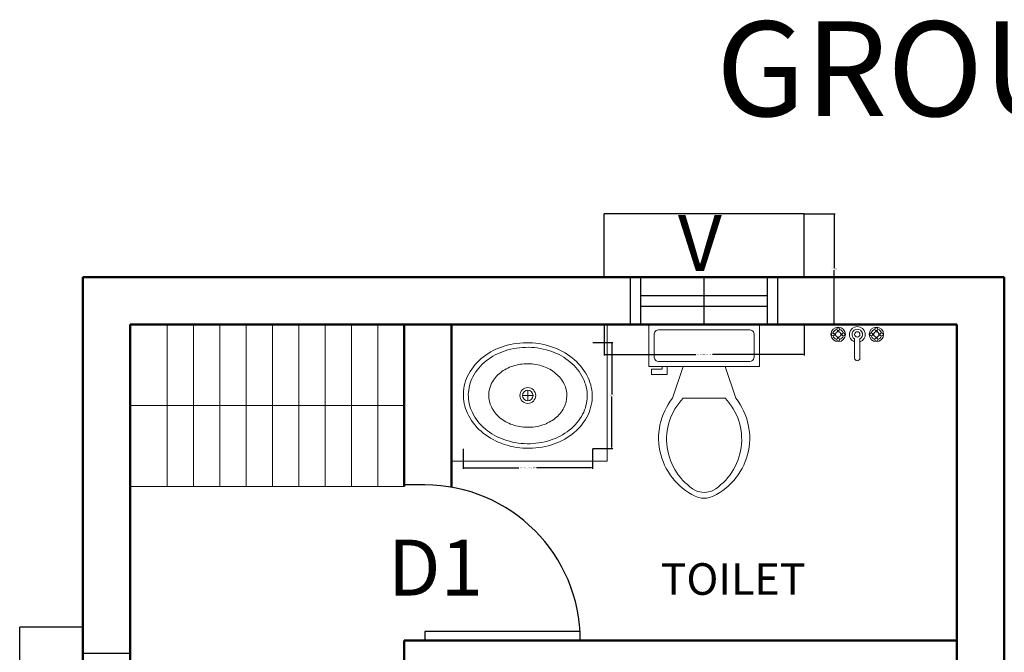
# Model space of a CAD drawing. Units: inches. Extents: x -105 to 1196, y -792 to 119.
# Tile 9 of 23: x -57 to 130, y -1 to 119. Entities that reach past the tile are written whole.
import ezdxf

# ---------------------------------------------------------------- set-up
doc = ezdxf.new("R2010")
doc.units = ezdxf.units.IN
doc.header["$MEASUREMENT"] = 0
for name, color, linetype, lineweight in [('A-ANNO-DIMS', 2, 'Continuous', 18), ('A-ANNO-TEXT', 7, 'Continuous', 25), ('A-AREA-IDEN', 7, 'Continuous', 25), ('A-DOOR', 4, 'Continuous', 25), ('A-FLOR-FIXT', 8, 'Continuous', 18), ('A-GLAZ', 4, 'Continuous', 25), ('A-WALL', 3, 'Continuous', 50)]:
    doc.layers.add(name, color=color, linetype=linetype, lineweight=lineweight)
doc.styles.get("Standard").update_dxf_attribs({"font": 'arial.ttf'})
doc.dimstyles.get("Standard").update_dxf_attribs({"dimtxt": 0.18, "dimasz": 0.18, "dimexe": 0.18, "dimexo": 0.0625, "dimgap": 0.09, "dimtad": 0, "dimtih": 1, "dimtoh": 1, "dimdec": 1, "dimzin": 0, "dimdsep": 46, "dimlunit": 4, "dimtxsty": 'Standard', "dimcen": 0.09, "dimadec": 0, "dimazin": 0, "dimtfac": 1, "dimtdec": 1, "dimtofl": 0, "dimtmove": 0, "dimatfit": 3, "dimfxl": 1, "dimtolj": 1, "dimtzin": 0, "dimarcsym": 0})

# ---------------------------------------------------------------- blocks, each defined once
blk = doc.blocks.new('*U2')
for p, q in [((-750, 0), (-750, -100)), ((0, 0), (0, -100))]:
    blk.add_line(p, q)
blk.add_lwpolyline([(0, 0), (0, 750), (-43.75, 750), (-43.75, 0)], close=True)
blk.add_arc((0, 0), 750, 90, 180)
blk = doc.blocks.new('Sink - Oval top')
for p, q in [((-1, 0), (1, 0)), ((0, 1), (0, -1))]:
    blk.add_line(p, q)
for points in [[(-12.23, 0.39, 0.117634), (-11.46, -3.36, 0.104469), (-8.88, -6.8, 0.090016), (-5.08, -9.07, 0.08192), (-0.32, -10.02, 0.08192), (4.49, -9.38, 0.090016), (8.42, -7.36, 0.104469), (11.22, -4.09, 0.117634), (12.23, -0.39, 0.117634), (11.46, 3.36, 0.104469), (8.88, 6.8, 0.090016), (5.08, 9.07, 0.08192), (0.32, 10.02, 0.08192), (-4.49, 9.38, 0.090016), (-8.42, 7.36, 0.104469), (-11.22, 4.09, 0.117634)], [(-11.29, 0.16, 0.118622), (-10.52, -3.25, 0.104678), (-8.07, -6.36, 0.089562), (-4.54, -8.37, 0.081185), (-0.13, -9.15, 0.081185), (4.3, -8.49, 0.089562), (7.89, -6.58, 0.104678), (10.42, -3.55, 0.118622), (11.29, -0.16, 0.118622), (10.52, 3.25, 0.104678), (8.07, 6.36, 0.089562), (4.54, 8.37, 0.081185), (0.13, 9.15, 0.081185), (-4.3, 8.49, 0.089562), (-7.89, 6.58, 0.104678), (-10.42, 3.55, 0.118622)], [(-7.42, 0.08, 0.118283), (-6.91, -2.17, 0.104607), (-5.29, -4.21, 0.089718), (-2.97, -5.53, 0.081436), (-0.07, -6.04, 0.081436), (2.84, -5.59, 0.089718), (5.2, -4.33, 0.104607), (6.86, -2.32, 0.118283), (7.42, -0.08, 0.118283), (6.91, 2.17, 0.104607), (5.29, 4.21, 0.089718), (2.97, 5.53, 0.081436), (0.07, 6.04, 0.081436), (-2.84, 5.59, 0.089718), (-5.2, 4.33, 0.104607), (-6.86, 2.32, 0.118283)]]:
    blk.add_lwpolyline(points, format="xyb", close=True)
for radius in [1.5, 1]:
    blk.add_circle((0, 0), radius)
blk = doc.blocks.new('Toilet - top')
for p, q in [((9.5, -6), (9.5, -2)), ((-10, -8.5), (-8, -8.5)), ((-10, -9.5), (-10, -8.5)), ((-8, -8.5), (-8, -8)), ((-7, -8), (-7, -9.5)), ((-4, -8), (-6, -14)), ((4, -8), (6, -14)), ((-7, -9.5), (-10, -9.5)), ((4, -14), (-4, -14))]:
    blk.add_line(p, q)
blk.add_lwpolyline([(10.5, -8), (10.5, 0), (-10.5, 0), (-10.5, -8)], close=True)
for points in [[(8.5, -1), (-8.5, -1)], [(-9.5, -2), (-9.5, -6)], [(-8.5, -7), (8.5, -7)]]:
    blk.add_lwpolyline(points)
for centre, radius, start, end in [((-8.62, -1.88), 0.884, 81.8699, 188.1301), ((8.62, -1.88), 0.884, 351.8699, 98.1301), ((-8.62, -6.12), 0.884, 171.8699, 278.1301), ((8.62, -6.12), 0.884, 261.8699, 8.1301), ((3.52, -21.58), 12.17, 141.4691, 247.9714), ((4.2, -21.82), 11.33, 136.3677, 238.9468), ((-3.52, -21.58), 12.17, 292.0284, 38.5307), ((-4.2, -21.82), 11.33, 301.053, 43.6321), ((0, -27.88), 4, 245.7318, 294.2682), ((0, -29), 4, 254.8605, 285.1395)]:
    blk.add_arc(centre, radius, start, end)
blk = doc.blocks.new('Faucet - Bathroom top')
for p, q in [((-4.107, 0.125), (-4.375, 0.125)), ((-3.75, 0.4788), (-3.75, 0.75)), ((-3.5, 0.482), (-3.5, 0.75)), ((-3.1461, 0.125), (-2.875, 0.125)), ((3.143, 0.125), (2.875, 0.125)), ((3.5, 0.4788), (3.5, 0.75)), ((3.75, 0.482), (3.75, 0.75)), ((4.1039, 0.125), (4.375, 0.125)), ((-4.1039, -0.125), (-4.375, -0.125)), ((-3.75, -0.4821), (-3.75, -0.75)), ((-3.5, -0.4789), (-3.5, -0.75)), ((-3.143, -0.125), (-2.875, -0.125)), ((-0.5, -0.8639), (-0.5, -4.5)), ((0.5, -4.5), (0.5, -0.8631)), ((3.1461, -0.125), (2.875, -0.125)), ((3.5, -0.4821), (3.5, -0.75)), ((3.75, -0.4789), (3.75, -0.75)), ((4.107, -0.125), (4.375, -0.125))]:
    blk.add_line(p, q)
for centre, radius in [((-3.625, 0), 1.375), ((-4.625, 0), 0.2795), ((-3.625, 0), 0.5), ((-3.625, 1), 0.2795), ((-2.625, 0), 0.2795), ((0, 0), 0.5), ((3.625, 0), 1.375), ((2.625, 0), 0.2795), ((3.625, 0), 0.5), ((3.625, 1), 0.2795), ((4.625, 0), 0.2795), ((-3.625, -1), 0.2795), ((3.625, -1), 0.2795)]:
    blk.add_circle(centre, radius)
for centre, radius, start, end in [((-3.625, 0), 1, 105.2407, 164.2093), ((-3.625, 0), 1, 16.44125, 74.07887), ((0, 0), 1.5, 289.6514, 250.3603), ((0, 0), 1, 300.3431, 239.7554), ((3.625, 0), 1, 106.12, 164.0884), ((3.625, 0), 1, 16.23422, 73.90469), ((-3.625, 0), 1, 196.2342, 253.9047), ((-3.625, 0), 1, 286.12, 344.0884), ((3.625, 0), 1, 196.4413, 254.0789), ((3.625, 0), 1, 285.2407, 344.2093), ((0, -4.5), 0.5, 180, 0)]:
    blk.add_arc(centre, radius, start, end)
blk = doc.blocks.new('WIN-1200')
at = {"ltscale": 2}
for p, q in [((12, 62), (0, 62)), ((0, 0), (0, 62)), ((12, 57), (12, 62)), ((12, 5), (12, 0)), ((12, 0), (0, 0))]:
    blk.add_line(p, q, dxfattribs=at)
for p, q in [((21, 57), (12, 57)), ((21, 5), (12, 5))]:
    blk.add_line(p, q)
blk = doc.blocks.new('VENT-600')
for p, q in [((0, 9), (0, 21)), ((38, 21), (0, 21)), ((38, 9), (38, 21)), ((5, 9), (0, 9)), ((5, 0), (5, 9)), ((33, 0), (33, 9)), ((33, 9), (38, 9))]:
    blk.add_line(p, q)
blk = doc.blocks.new('*D57')
at = {"layer": 'A-ANNO-DIMS', "color": 0, "lineweight": -2, "transparency": 16777216}
for p, q in [((53.74, 60.71), (53.74, 54.89)), ((91.74, 60.71), (91.74, 54.89)), ((53.92, 55.07), (71.16, 55.07)), ((91.56, 55.07), (74.33, 55.07))]:
    blk.add_line(p, q, dxfattribs=at)
at = {"layer": 'A-ANNO-DIMS', "color": 0, "transparency": 16777216}
for points in [[(53.92, 55.1), (53.92, 55.04), (53.74, 55.07)], [(91.56, 55.1), (91.56, 55.04), (91.74, 55.07)]]:
    blk.add_solid(points, dxfattribs=at)
at = {"layer": 'Defpoints', "color": 0, "transparency": 16777216}
for p in [(53.74, 60.77), (91.74, 60.77), (91.74, 55.07)]:
    blk.add_point(p, dxfattribs=at)
at = {"layer": 'A-ANNO-DIMS', "color": 0, "transparency": 16777216, "insert": (72.74, 55.07), "char_height": 0.18, "attachment_point": 5}
blk.add_mtext('\\A1;VENTILATOR V 3\'-2" TYP.', dxfattribs=at)
blk = doc.blocks.new('*D58')
at = {"layer": 'A-ANNO-DIMS', "color": 0, "lineweight": -2, "transparency": 16777216}
for p, q in [((91.81, 81.77), (97.62, 81.77)), ((97.44, 81.59), (97.44, 71.45)), ((97.44, 60.95), (97.44, 71.09)), ((91.81, 60.77), (97.62, 60.77))]:
    blk.add_line(p, q, dxfattribs=at)
at = {"layer": 'A-ANNO-DIMS', "color": 0, "transparency": 16777216}
for points in [[(97.41, 81.59), (97.47, 81.59), (97.44, 81.77)], [(97.41, 60.95), (97.47, 60.95), (97.44, 60.77)]]:
    blk.add_solid(points, dxfattribs=at)
at = {"layer": 'Defpoints', "color": 0, "transparency": 16777216}
for p in [(91.74, 81.77), (97.44, 81.77), (91.74, 60.77)]:
    blk.add_point(p, dxfattribs=at)
at = {"layer": 'A-ANNO-DIMS', "color": 0, "transparency": 16777216, "insert": (97.44, 71.27), "char_height": 0.18, "attachment_point": 5}
blk.add_mtext('\\A1;1\'-9" TYP.', dxfattribs=at)
blk = doc.blocks.new('*D63')
at = {"layer": 'A-ANNO-DIMS', "color": 0, "lineweight": -2, "transparency": 16777216}
for p, q in [((26.96, 37.16), (26.96, 33.36)), ((51.51, 37.16), (51.51, 33.36)), ((27.14, 33.54), (37.56, 33.54)), ((51.33, 33.54), (40.91, 33.54))]:
    blk.add_line(p, q, dxfattribs=at)
at = {"layer": 'A-ANNO-DIMS', "color": 0, "transparency": 16777216}
for points in [[(27.14, 33.57), (27.14, 33.51), (26.96, 33.54)], [(51.33, 33.57), (51.33, 33.51), (51.51, 33.54)]]:
    blk.add_solid(points, dxfattribs=at)
at = {"layer": 'Defpoints', "color": 0, "transparency": 16777216}
for p in [(26.96, 37.22), (51.51, 37.22), (51.51, 33.54)]:
    blk.add_point(p, dxfattribs=at)
at = {"layer": 'A-ANNO-DIMS', "color": 0, "transparency": 16777216, "insert": (39.24, 33.54), "char_height": 0.18, "attachment_point": 5}
blk.add_mtext('\\A1;WASH BASIN 2\'-0 1/2" TYP.', dxfattribs=at)
blk = doc.blocks.new('*D64')
at = {"layer": 'A-ANNO-DIMS', "color": 0, "lineweight": -2, "transparency": 16777216}
for p, q in [((51.57, 57.36), (55.37, 57.36)), ((55.19, 57.18), (55.19, 47.47)), ((55.19, 37.4), (55.19, 47.11)), ((51.57, 37.22), (55.37, 37.22))]:
    blk.add_line(p, q, dxfattribs=at)
at = {"layer": 'A-ANNO-DIMS', "color": 0, "transparency": 16777216}
for points in [[(55.16, 57.18), (55.22, 57.18), (55.19, 57.36)], [(55.16, 37.4), (55.22, 37.4), (55.19, 37.22)]]:
    blk.add_solid(points, dxfattribs=at)
at = {"layer": 'Defpoints', "color": 0, "transparency": 16777216}
for p in [(51.51, 57.36), (55.19, 57.36), (51.51, 37.22)]:
    blk.add_point(p, dxfattribs=at)
at = {"layer": 'A-ANNO-DIMS', "color": 0, "transparency": 16777216, "insert": (55.19, 47.29), "char_height": 0.18, "attachment_point": 5}
blk.add_mtext('\\A1;1\'-8" TYP.', dxfattribs=at)

msp = doc.modelspace()

# ---------------------------------------------------------------- linework, layer by layer
at = {"layer": 'A-FLOR-FIXT'}
for p, q in [((-29.26, 30.04), (-29.26, 60.77)), ((-24.26, 30.04), (-24.26, 60.77)), ((-19.26, 30.04), (-19.26, 60.77)), ((-14.26, 30.04), (-14.26, 60.77)), ((-9.26, 30.04), (-9.26, 60.77)), ((-4.26, 30.04), (-4.26, 60.77)), ((0.74, 30.04), (0.74, 60.77)), ((5.74, 30.04), (5.74, 60.77)), ((10.74, 30.04), (10.74, 60.77)), ((54.3, 34.79), (54.3, 60.77)), ((15.74, 45.4), (-36.26, 45.4)), ((24.74, 34.79), (54.3, 34.79)), ((15.74, 30.04), (-36.26, 30.04))]:
    msp.add_line(p, q, dxfattribs=at)
at = {"layer": 'A-GLAZ'}
for p, q in [((60.74, 60.77), (60.74, 69.77)), ((72.74, 60.77), (72.74, 69.77)), ((84.74, 60.77), (84.74, 69.77)), ((60.74, 66.27), (84.74, 66.27)), ((60.74, 64.27), (84.74, 64.27))]:
    msp.add_line(p, q, dxfattribs=at)
at = {"layer": 'A-WALL'}
for p, q in [((-45.26, 69.77), (129.74, 69.77)), ((-45.26, 69.77), (-45.26, -125.23)), ((129.74, 69.77), (129.74, -57.23)), ((-36.26, 60.77), (24.74, 60.77)), ((-36.26, 60.77), (-36.26, -116.23)), ((15.74, 30.04), (15.74, 60.77)), ((24.74, 29.86), (24.74, 60.77)), ((24.74, 29.86), (24.74, 60.77)), ((24.74, 60.77), (120.74, 60.77)), ((120.74, 60.77), (120.74, -76.34)), ((120.74, 60.77), (120.74, 0.77)), ((48.74, 0.77), (15.74, 0.77)), ((15.74, -8.23), (15.74, 0.77)), ((120.74, 0.77), (48.74, 0.77))]:
    msp.add_line(p, q, dxfattribs=at)

# ---------------------------------------------------------------- block references
at = {"layer": 'A-DOOR', "xscale": 0.0393700787401575, "yscale": 0.0393700787401575, "zscale": 0.0393700787401575, "rotation": 270}
msp.add_blockref('*U2', (19.68, 0.77), dxfattribs=at)
at = {"layer": 'A-FLOR-FIXT'}
for name, p in [('Toilet - top', (72.74, 60.77)), ('Faucet - Bathroom top', (101.82, 58.89)), ('Sink - Oval top', (39.24, 47.29))]:
    msp.add_blockref(name, p, dxfattribs=at)
at = {"layer": 'A-GLAZ'}
for name, p in [('VENT-600', (53.74, 60.77)), ('WIN-1200', (-57.26, -58.73))]:
    msp.add_blockref(name, p, dxfattribs=at)

# ---------------------------------------------------------------- texts
at = {"layer": 'A-ANNO-TEXT'}
for s, height, p in [('GROUND  FLOOR  PLAN', 18, (75.01, 100.34)), ('V', 10.64, (67.75, 70.96)), ('D1', 10.636, (12.7, 9.29))]:
    msp.add_text(s, height=height, dxfattribs=at).set_placement(p)
at = {"layer": 'A-AREA-IDEN', "insert": (64.47, 15.44), "char_height": 6, "attachment_point": 1}
msp.add_mtext_dynamic_manual_height_columns('TOILET', width=59.5623, gutter_width=1, heights=[0], dxfattribs=at)

# ---------------------------------------------------------------- dimensions: what is measured, and where the dimension line sits
at = {"layer": 'A-ANNO-DIMS'}
for base, p1, p2, picture, middle in [((97.44, 81.77), (91.74, 60.77), (91.74, 81.77), '*D58', (97.44, 71.27)), ((55.19, 57.36), (51.51, 37.22), (51.51, 57.36), '*D64', (55.19, 47.29))]:
    dim = msp.add_linear_dim(base=base, p1=p1, p2=p2, angle=90, text='<> TYP.', dimstyle='Standard', override={"dimdec": 1, "dimlfac": 1, "dimrnd": 0, "dimzin": 1, "dimdsep": 46, "dimlunit": 4, "dimfrac": 2}, dxfattribs=at)
    dim.commit()
    dim.dimension.update_dxf_attribs({"geometry": picture, "text_midpoint": middle})
for base, p1, p2, text, picture, middle in [((91.74, 55.07), (53.74, 60.77), (91.74, 60.77), 'VENTILATOR V <> TYP.', '*D57', (72.74, 55.07)), ((51.5106, 33.5375), (26.9597, 37.2201), (51.5106, 37.2201), 'WASH BASIN <> TYP.', '*D63', (39.2351, 33.5375))]:
    dim = msp.add_linear_dim(base=base, p1=p1, p2=p2, text=text, dimstyle='Standard', override={"dimdec": 1, "dimlfac": 1, "dimrnd": 0, "dimzin": 1, "dimdsep": 46, "dimlunit": 4, "dimfrac": 2}, dxfattribs=at)
    dim.commit()
    dim.dimension.update_dxf_attribs({"geometry": picture, "text_midpoint": middle})

doc.saveas('drawing.dxf')
